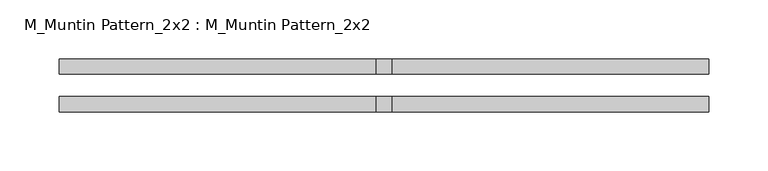
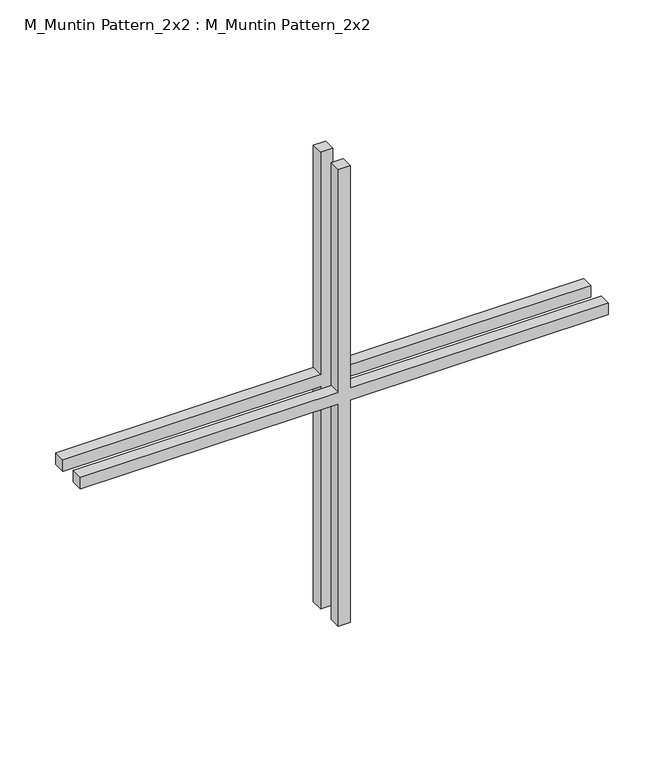
"""IFC4 building model written with IfcOpenShell, lengths in millimetres: proxy geometry, M_Muntin Pattern_2x2 : M_Muntin Pattern_2x2."""

from ifc_helpers import new_model, si_unit, frame, origin, place, context, project, spatial, polyline, outline, extrude, source, transform, mapped, element, save


def m_muntin_pattern_2x2_m_muntin_pattern_2x2_8c828626(model_context):
    return source(origin(), model_context, "Body", "SweptSolid", [
        extrude(outline(polyline([(257.1375, -6.35), (257.1375, -273.8), (244.4375, -273.8), (244.4375, -6.35), (0.0, -6.35), (0.0, 6.35), (244.4375, 6.35), (244.4375, 273.8), (257.1375, 273.8), (257.1375, 6.35), (501.575, 6.35), (501.575, -6.35), (257.1375, -6.35)])), frame((0.0, 9.525, 0.0), z_axis=(0.0, 1.0, 0.0), x_axis=(0.0, 0.0, 1.0)), (0.0, 0.0, 1.0), 12.7),
        extrude(outline(polyline([(257.1375, -6.35), (257.1375, -273.8), (244.4375, -273.8), (244.4375, -6.35), (0.0, -6.35), (0.0, 6.35), (244.4375, 6.35), (244.4375, 273.8), (257.1375, 273.8), (257.1375, 6.35), (501.575, 6.35), (501.575, -6.35), (257.1375, -6.35)])), frame((0.0, -22.225, 0.0), z_axis=(0.0, 1.0, 0.0), x_axis=(0.0, 0.0, 1.0)), (0.0, 0.0, 1.0), 12.7),
    ])


if __name__ == "__main__":
    model = new_model("IFC4")
    model_context = context("Model", 3, world=origin())
    ifc_project = project(units=[si_unit("LENGTHUNIT", "METRE", prefix="MILLI")], contexts=[model_context])
    site = spatial("IfcSite", under=ifc_project)
    building = spatial("IfcBuilding", under=site)
    placement = place(None, origin())
    m_muntin_pattern_2x2_m_muntin_pattern_2x2_shape = m_muntin_pattern_2x2_m_muntin_pattern_2x2_8c828626(model_context)
    element("IfcBuildingElementProxy", 1, Name="M_Muntin Pattern_2x2 : M_Muntin Pattern_2x2", ObjectType="M_Muntin Pattern_2x2 : M_Muntin Pattern_2x2", at=placement, inside=building, context=model_context, shape_type="MappedRepresentation", body=[
        mapped(m_muntin_pattern_2x2_m_muntin_pattern_2x2_shape, transform((0.0, 0.0, 0.0), x_axis=(1.0, 0.0, 0.0), y_axis=(0.0, 1.0, 0.0), z_axis=(0.0, 0.0, 1.0))),
    ])
    save(model, "model.ifc")

# Revit data of these elements
# Type "M_Muntin Pattern_2x2 : M_Muntin Pattern_2x2"
#   Width [instance default] = 1200 mm
#   Thickness = 12.7 mm
#   Height [instance default] = 1200 mm
#   Distance = 19.05 mm
#   Interior Material [instance default] = none
#   Exterior Material [instance default] = none
#   Default Elevation = 0
# Element 1 (IfcBuildingElementProxy, "M_Muntin Pattern_2x2 : M_Muntin Pattern_2x2")
#   Width = 547.6 mm
#   Height = 501.575 mm
#   Interior Material = Wood - Stained
#   Exterior Material = Clad - White
#   Materials on its faces: "Clad - White", "Wood - Stained"
# Materials
#   "Clad - White": class "Wood", colour RGB 245 245 243, transparency 0, Cost = 0
#   "Wood - Stained": class "Wood", colour RGB 173 132 96, transparency 0, Cost = 0
